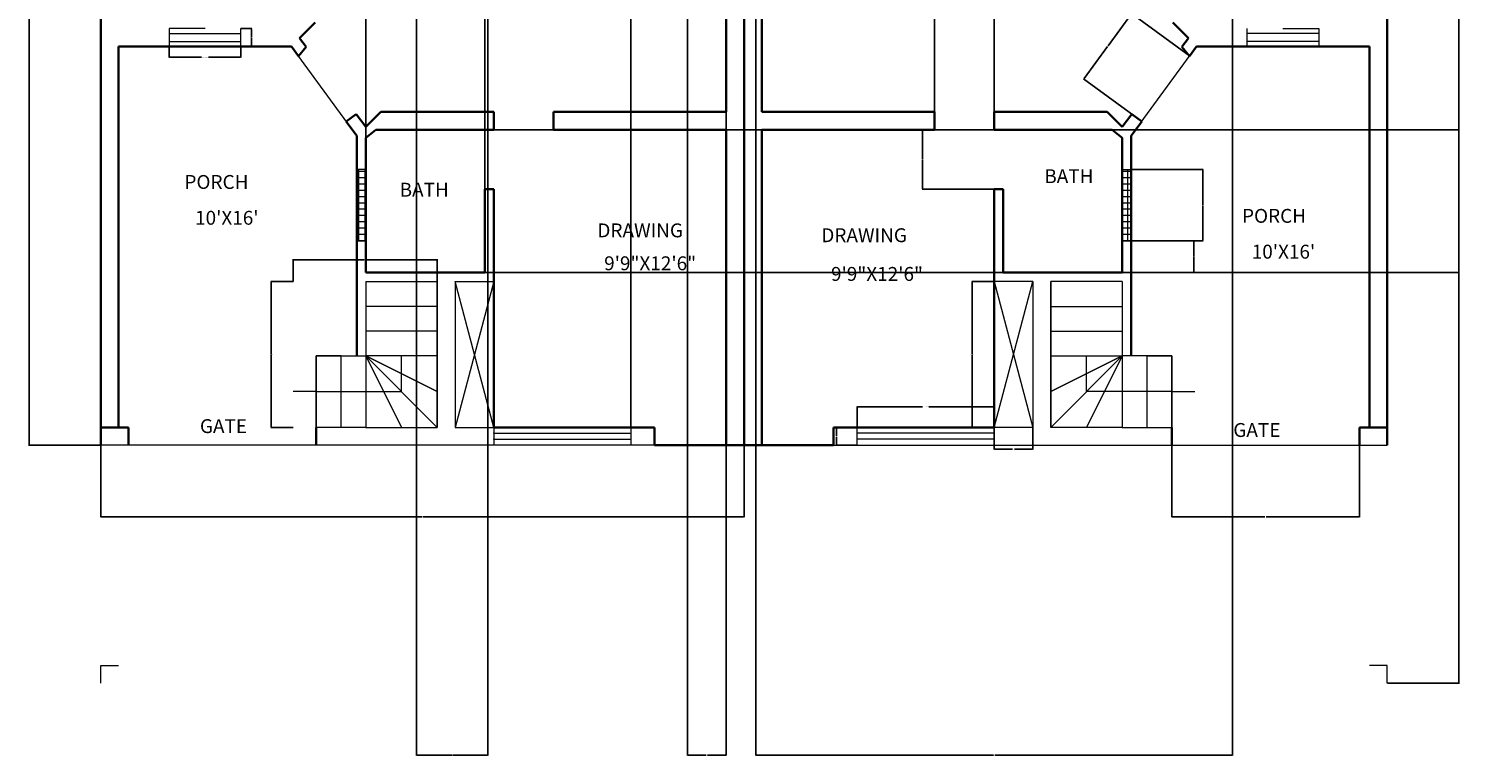
# Model space of a CAD drawing. Units: millimetres. Extents: x 2218 to 2939, y 1369 to 2162.
# Tile 1 of 2: x 2218 to 2939, y 1369 to 1736. Entities that reach past the tile are written whole.
import ezdxf

# ---------------------------------------------------------------- set-up
doc = ezdxf.new("R2010")
doc.units = ezdxf.units.MM
for name, color, linetype, lineweight in [('A-ANNO-DIMS', 2, 'Continuous', 18), ('A-ANNO-TEXT', 7, 'Continuous', 18), ('A-AREA-IDEN', 7, 'Continuous', 25), ('A-DOOR', 3, 'Continuous', 18), ('A-FLOR-CASE', 9, 'Continuous', 18), ('A-FLOR-STRS', 2, 'Continuous', 18), ('A-GLAZ', 4, 'Continuous', 18), ('A-GLAZ-PATT', 252, 'Continuous', 13), ('A-REFR-NODE', 8, 'Continuous', 13), ('A-WALL', 7, 'Continuous', 35), ('C-PROP', 8, 'Continuous', 18)]:
    doc.layers.add(name, color=color, linetype=linetype, lineweight=lineweight)
doc.styles.get("Standard").update_dxf_attribs({"font": 'arial.ttf'})
doc.dimstyles.get("Standard").update_dxf_attribs({"dimtxt": 0.18, "dimasz": 0.18, "dimexe": 0.18, "dimexo": 0.0625, "dimgap": 0.09, "dimtad": 0, "dimtih": 1, "dimtoh": 1, "dimdec": 4, "dimzin": 0, "dimdsep": 46, "dimtxsty": 'Standard', "dimcen": 0.09, "dimadec": 0, "dimazin": 0, "dimtfac": 1, "dimtdec": 4, "dimtofl": 0, "dimtmove": 0, "dimatfit": 3, "dimfxl": 1, "dimtolj": 1, "dimtzin": 0, "dimarcsym": 0})

# ---------------------------------------------------------------- blocks, each defined once
blk = doc.blocks.new('WIN-KITCHEN-PORCH')
for p, q in [((18, 9), (0, 9)), ((0, 9), (0, 0)), ((36, 0), (36, 9)), ((0, 6.5), (36, 6.5)), ((0, 2.5), (36, 2.5)), ((0, 0), (36, 0))]:
    blk.add_line(p, q)
blk = doc.blocks.new('WIN-DRAWING-FRONT')
for p, q in [((0, 9), (0, 0)), ((69, 9), (69, 0)), ((0, 6), (69, 6)), ((0, 3), (69, 3))]:
    blk.add_line(p, q)
blk = doc.blocks.new('STAIR-PORCH-WINDER')
for p, q in [((36.6, 73.5), (72.6, 73.5)), ((36.6, 73.5), (72.6, 73.5)), ((36.6, 73.5), (36.6, 0)), ((72.6, 73.5), (72.6, 0)), ((72.6, 36), (72.6, 73.5)), ((72.6, 61), (36.6, 61)), ((72.6, 48.5), (36.6, 48.5)), ((24.1, 36), (11.6, 36)), ((11.6, 36), (11.6, 0)), ((11.6, 0), (11.6, 36)), ((11.6, 36), (32.1, 36)), ((24.1, 0), (24.1, 36)), ((32.1, 36), (36.6, 36)), ((72.6, 36), (36.6, 36)), ((36.6, 36), (72.6, 18)), ((72.6, 18), (36.6, 36)), ((36.6, 36), (54.6, 0)), ((36.6, 36), (72.6, 0)), ((54.6, 18), (54.6, 36)), ((72.6, 0), (72.6, 36)), ((11.6, 18), (0, 18)), ((11.6, 18), (54.6, 18)), ((32.1, 0), (11.6, 0)), ((36.6, 0), (24.1, 0)), ((36.6, 0), (72.6, 0))]:
    blk.add_line(p, q)
blk = doc.blocks.new('CASEWORK-DRAWING')
for p, q in [((0, 73.5), (0, 0)), ((19.5, 0), (0, 73.5)), ((0, 73.5), (19.5, 73.5)), ((19.5, 73.5), (0, 0)), ((0, 73.5), (19.5, 73.5)), ((0, 0), (19.5, 0))]:
    blk.add_line(p, q)
blk = doc.blocks.new('*D15')
at = {"layer": 'A-ANNO-DIMS', "color": 0, "lineweight": -2, "transparency": 16777216}
for p, q in [((2288.88, 1726.51), (2288.88, 1721)), ((2324.88, 1726.51), (2324.88, 1721)), ((2289.06, 1721.18), (2305.18, 1721.18)), ((2324.7, 1721.18), (2308.58, 1721.18))]:
    blk.add_line(p, q, dxfattribs=at)
at = {"layer": 'A-ANNO-DIMS', "color": 0, "transparency": 16777216}
for points in [[(2289.06, 1721.21), (2289.06, 1721.15), (2288.88, 1721.18)], [(2324.7, 1721.21), (2324.7, 1721.15), (2324.88, 1721.18)]]:
    blk.add_solid(points, dxfattribs=at)
at = {"layer": 'Defpoints', "color": 0, "transparency": 16777216}
for p in [(2288.88, 1726.58), (2324.88, 1726.58), (2324.88, 1721.18)]:
    blk.add_point(p, dxfattribs=at)
at = {"layer": 'A-ANNO-DIMS', "color": 0, "transparency": 16777216, "insert": (2306.88, 1721.18), "char_height": 0.18, "attachment_point": 5}
blk.add_mtext('\\A1;KITCHEN WINDOW 36 TYP.', dxfattribs=at)
blk = doc.blocks.new('*D16')
at = {"layer": 'A-ANNO-DIMS', "color": 0, "lineweight": -2, "transparency": 16777216}
for p, q in [((2324.94, 1735.58), (2330.46, 1735.58)), ((2330.28, 1735.4), (2330.28, 1731.26)), ((2330.28, 1726.76), (2330.28, 1730.89)), ((2324.94, 1726.58), (2330.46, 1726.58))]:
    blk.add_line(p, q, dxfattribs=at)
at = {"layer": 'A-ANNO-DIMS', "color": 0, "transparency": 16777216}
for points in [[(2330.25, 1735.4), (2330.31, 1735.4), (2330.28, 1735.58)], [(2330.25, 1726.76), (2330.31, 1726.76), (2330.28, 1726.58)]]:
    blk.add_solid(points, dxfattribs=at)
at = {"layer": 'Defpoints', "color": 0, "transparency": 16777216}
for p in [(2324.88, 1735.58), (2330.28, 1735.58), (2324.88, 1726.58)]:
    blk.add_point(p, dxfattribs=at)
at = {"layer": 'A-ANNO-DIMS', "color": 0, "transparency": 16777216, "insert": (2330.28, 1731.08), "char_height": 0.18, "attachment_point": 5}
blk.add_mtext('\\A1;9 TYP.', dxfattribs=at)
blk = doc.blocks.new('*D17')
at = {"layer": 'A-ANNO-DIMS', "color": 0, "lineweight": -2, "transparency": 16777216}
for p, q in [((2635.38, 1534.64), (2635.38, 1545.11)), ((2635.56, 1544.93), (2668.3, 1544.93)), ((2704.2, 1544.93), (2671.46, 1544.93)), ((2704.38, 1534.64), (2704.38, 1545.11))]:
    blk.add_line(p, q, dxfattribs=at)
at = {"layer": 'A-ANNO-DIMS', "color": 0, "transparency": 16777216}
for points in [[(2635.56, 1544.96), (2635.56, 1544.9), (2635.38, 1544.93)], [(2704.2, 1544.96), (2704.2, 1544.9), (2704.38, 1544.93)]]:
    blk.add_solid(points, dxfattribs=at)
at = {"layer": 'Defpoints', "color": 0, "transparency": 16777216}
for p in [(2635.38, 1544.93), (2635.38, 1534.58), (2704.38, 1534.58)]:
    blk.add_point(p, dxfattribs=at)
at = {"layer": 'A-ANNO-DIMS', "color": 0, "transparency": 16777216, "insert": (2669.88, 1544.93), "char_height": 0.18, "attachment_point": 5}
blk.add_mtext('\\A1;FRONT WINDOW 69 TYP.', dxfattribs=at)
blk = doc.blocks.new('*D18')
at = {"layer": 'A-ANNO-DIMS', "color": 0, "lineweight": -2, "transparency": 16777216}
for p, q in [((2635.32, 1534.58), (2624.85, 1534.58)), ((2625.03, 1534.4), (2625.03, 1530.26)), ((2625.03, 1525.76), (2625.03, 1529.89)), ((2635.32, 1525.58), (2624.85, 1525.58))]:
    blk.add_line(p, q, dxfattribs=at)
at = {"layer": 'A-ANNO-DIMS', "color": 0, "transparency": 16777216}
for points in [[(2625, 1534.4), (2625.06, 1534.4), (2625.03, 1534.58)], [(2625, 1525.76), (2625.06, 1525.76), (2625.03, 1525.58)]]:
    blk.add_solid(points, dxfattribs=at)
at = {"layer": 'Defpoints', "color": 0, "transparency": 16777216}
for p in [(2635.38, 1534.58), (2625.03, 1525.58), (2635.38, 1525.58)]:
    blk.add_point(p, dxfattribs=at)
at = {"layer": 'A-ANNO-DIMS', "color": 0, "transparency": 16777216, "insert": (2625.03, 1530.08), "char_height": 0.18, "attachment_point": 5}
blk.add_mtext('\\A1;9 TYP.', dxfattribs=at)
blk = doc.blocks.new('*D19')
at = {"layer": 'A-ANNO-DIMS', "color": 0, "lineweight": -2, "transparency": 16777216}
for p, q in [((2351.22, 1608.08), (2340.08, 1608.08)), ((2340.26, 1607.9), (2340.26, 1571.51)), ((2340.26, 1534.76), (2340.26, 1571.14)), ((2351.22, 1534.58), (2340.08, 1534.58))]:
    blk.add_line(p, q, dxfattribs=at)
at = {"layer": 'A-ANNO-DIMS', "color": 0, "transparency": 16777216}
for points in [[(2340.23, 1607.9), (2340.29, 1607.9), (2340.26, 1608.08)], [(2340.23, 1534.76), (2340.29, 1534.76), (2340.26, 1534.58)]]:
    blk.add_solid(points, dxfattribs=at)
at = {"layer": 'Defpoints', "color": 0, "transparency": 16777216}
for p in [(2340.26, 1608.08), (2351.28, 1608.08), (2351.28, 1534.58)]:
    blk.add_point(p, dxfattribs=at)
at = {"layer": 'A-ANNO-DIMS', "color": 0, "transparency": 16777216, "insert": (2340.26, 1571.33), "char_height": 0.18, "attachment_point": 5}
blk.add_mtext('\\A1;PORCH STAIR 74 TYP.', dxfattribs=at)
blk = doc.blocks.new('*D20')
at = {"layer": 'A-ANNO-DIMS', "color": 0, "lineweight": -2, "transparency": 16777216}
for p, q in [((2351.28, 1608.14), (2351.28, 1619.28)), ((2351.46, 1619.1), (2387.05, 1619.1)), ((2423.7, 1619.1), (2388.11, 1619.1)), ((2423.88, 1608.14), (2423.88, 1619.28))]:
    blk.add_line(p, q, dxfattribs=at)
at = {"layer": 'A-ANNO-DIMS', "color": 0, "transparency": 16777216}
for points in [[(2351.46, 1619.13), (2351.46, 1619.07), (2351.28, 1619.1)], [(2423.7, 1619.13), (2423.7, 1619.07), (2423.88, 1619.1)]]:
    blk.add_solid(points, dxfattribs=at)
at = {"layer": 'Defpoints', "color": 0, "transparency": 16777216}
for p in [(2423.88, 1619.1), (2351.28, 1608.08), (2423.88, 1608.08)]:
    blk.add_point(p, dxfattribs=at)
at = {"layer": 'A-ANNO-DIMS', "color": 0, "transparency": 16777216, "insert": (2387.58, 1619.1), "char_height": 0.18, "attachment_point": 5}
blk.add_mtext('\\A1;73 TYP.', dxfattribs=at)
blk = doc.blocks.new('*D23')
at = {"layer": 'A-ANNO-DIMS', "color": 0, "lineweight": -2, "transparency": 16777216}
for p, q in [((2704.32, 1608.08), (2693.17, 1608.08)), ((2693.35, 1607.9), (2693.35, 1571.51)), ((2693.35, 1534.76), (2693.35, 1571.14)), ((2704.32, 1534.58), (2693.17, 1534.58))]:
    blk.add_line(p, q, dxfattribs=at)
at = {"layer": 'A-ANNO-DIMS', "color": 0, "transparency": 16777216}
for points in [[(2693.32, 1607.9), (2693.38, 1607.9), (2693.35, 1608.08)], [(2693.32, 1534.76), (2693.38, 1534.76), (2693.35, 1534.58)]]:
    blk.add_solid(points, dxfattribs=at)
at = {"layer": 'Defpoints', "color": 0, "transparency": 16777216}
for p in [(2693.35, 1608.08), (2704.38, 1608.08), (2704.38, 1534.58)]:
    blk.add_point(p, dxfattribs=at)
at = {"layer": 'A-ANNO-DIMS', "color": 0, "transparency": 16777216, "insert": (2693.35, 1571.33), "char_height": 0.18, "attachment_point": 5}
blk.add_mtext('\\A1;CASEWORK 74 TYP.', dxfattribs=at)
blk = doc.blocks.new('*D24')
at = {"layer": 'A-ANNO-DIMS', "color": 0, "lineweight": -2, "transparency": 16777216}
for p, q in [((2704.38, 1534.51), (2704.38, 1523.37)), ((2723.88, 1534.51), (2723.88, 1523.37)), ((2704.56, 1523.55), (2713.6, 1523.55)), ((2723.7, 1523.55), (2714.66, 1523.55))]:
    blk.add_line(p, q, dxfattribs=at)
at = {"layer": 'A-ANNO-DIMS', "color": 0, "transparency": 16777216}
for points in [[(2704.56, 1523.58), (2704.56, 1523.52), (2704.38, 1523.55)], [(2723.7, 1523.58), (2723.7, 1523.52), (2723.88, 1523.55)]]:
    blk.add_solid(points, dxfattribs=at)
at = {"layer": 'Defpoints', "color": 0, "transparency": 16777216}
for p in [(2704.38, 1534.58), (2723.88, 1534.58), (2704.38, 1523.55)]:
    blk.add_point(p, dxfattribs=at)
at = {"layer": 'A-ANNO-DIMS', "color": 0, "transparency": 16777216, "insert": (2714.13, 1523.55), "char_height": 0.18, "attachment_point": 5}
blk.add_mtext('\\A1;20 TYP.', dxfattribs=at)
blk = doc.blocks.new('*D26')
at = {"layer": 'A-ANNO-DIMS', "color": 0, "lineweight": -2, "transparency": 16777216}
for p, q in [((2254.38, 1525.51), (2254.38, 1489.25)), ((2578.38, 1525.51), (2578.38, 1489.25)), ((2254.56, 1489.43), (2416.09, 1489.43)), ((2578.2, 1489.43), (2416.67, 1489.43))]:
    blk.add_line(p, q, dxfattribs=at)
at = {"layer": 'A-ANNO-DIMS', "color": 0, "transparency": 16777216}
for points in [[(2254.56, 1489.46), (2254.56, 1489.4), (2254.38, 1489.43)], [(2578.2, 1489.46), (2578.2, 1489.4), (2578.38, 1489.43)]]:
    blk.add_solid(points, dxfattribs=at)
at = {"layer": 'Defpoints', "color": 0, "transparency": 16777216}
for p in [(2254.38, 1525.58), (2578.38, 1525.58), (2254.38, 1489.43)]:
    blk.add_point(p, dxfattribs=at)
at = {"layer": 'A-ANNO-DIMS', "color": 0, "transparency": 16777216, "insert": (2416.38, 1489.43), "char_height": 0.18, "attachment_point": 5}
blk.add_mtext('\\A1;324', dxfattribs=at)
blk = doc.blocks.new('*D27')
at = {"layer": 'A-ANNO-DIMS', "color": 0, "lineweight": -2, "transparency": 16777216}
for p, q in [((2902.44, 2125.58), (2938.71, 2125.58)), ((2938.53, 2125.4), (2938.53, 1765.76)), ((2938.53, 1405.76), (2938.53, 1765.39)), ((2902.44, 1405.58), (2938.71, 1405.58))]:
    blk.add_line(p, q, dxfattribs=at)
at = {"layer": 'A-ANNO-DIMS', "color": 0, "transparency": 16777216}
for points in [[(2938.5, 2125.4), (2938.56, 2125.4), (2938.53, 2125.58)], [(2938.5, 1405.76), (2938.56, 1405.76), (2938.53, 1405.58)]]:
    blk.add_solid(points, dxfattribs=at)
at = {"layer": 'Defpoints', "color": 0, "transparency": 16777216}
for p in [(2902.38, 2125.58), (2938.53, 2125.58), (2902.38, 1405.58)]:
    blk.add_point(p, dxfattribs=at)
at = {"layer": 'A-ANNO-DIMS', "color": 0, "transparency": 16777216, "insert": (2938.53, 1765.58), "char_height": 0.18, "attachment_point": 5}
blk.add_mtext('\\A1;720', dxfattribs=at)
blk = doc.blocks.new('*D28')
at = {"layer": 'A-ANNO-DIMS', "color": 0, "lineweight": -2, "transparency": 16777216}
for p, q in [((2254.32, 2125.58), (2218.05, 2125.58)), ((2218.23, 2125.4), (2218.23, 1825.76)), ((2218.23, 1525.76), (2218.23, 1825.39)), ((2254.32, 1525.58), (2218.05, 1525.58))]:
    blk.add_line(p, q, dxfattribs=at)
at = {"layer": 'A-ANNO-DIMS', "color": 0, "transparency": 16777216}
for points in [[(2218.2, 2125.4), (2218.26, 2125.4), (2218.23, 2125.58)], [(2218.2, 1525.76), (2218.26, 1525.76), (2218.23, 1525.58)]]:
    blk.add_solid(points, dxfattribs=at)
at = {"layer": 'Defpoints', "color": 0, "transparency": 16777216}
for p in [(2218.23, 2125.58), (2254.38, 2125.58), (2254.38, 1525.58)]:
    blk.add_point(p, dxfattribs=at)
at = {"layer": 'A-ANNO-DIMS', "color": 0, "transparency": 16777216, "insert": (2218.23, 1825.58), "char_height": 0.18, "attachment_point": 5}
blk.add_mtext('\\A1;600', dxfattribs=at)
blk = doc.blocks.new('*D29')
at = {"layer": 'A-ANNO-DIMS', "color": 0, "lineweight": -2, "transparency": 16777216}
for p, q in [((2584.38, 2119.51), (2584.38, 1369.25)), ((2824.38, 2119.51), (2824.38, 1369.25)), ((2584.56, 1369.43), (2704.09, 1369.43)), ((2824.2, 1369.43), (2704.67, 1369.43))]:
    blk.add_line(p, q, dxfattribs=at)
at = {"layer": 'A-ANNO-DIMS', "color": 0, "transparency": 16777216}
for points in [[(2584.56, 1369.46), (2584.56, 1369.4), (2584.38, 1369.43)], [(2824.2, 1369.46), (2824.2, 1369.4), (2824.38, 1369.43)]]:
    blk.add_solid(points, dxfattribs=at)
at = {"layer": 'Defpoints', "color": 0, "transparency": 16777216}
for p in [(2584.38, 2119.58), (2824.38, 2119.58), (2824.38, 1369.43)]:
    blk.add_point(p, dxfattribs=at)
at = {"layer": 'A-ANNO-DIMS', "color": 0, "transparency": 16777216, "insert": (2704.38, 1369.43), "char_height": 0.18, "attachment_point": 5}
blk.add_mtext('\\A1;240', dxfattribs=at)
blk = doc.blocks.new('*D31')
at = {"layer": 'A-ANNO-DIMS', "color": 0, "lineweight": -2, "transparency": 16777216}
for p, q in [((2387.88, 1612.64), (2387.88, 2161.91)), ((2388.06, 2161.73), (2417.66, 2161.73)), ((2447.7, 2161.73), (2418.1, 2161.73)), ((2447.88, 1612.64), (2447.88, 2161.91))]:
    blk.add_line(p, q, dxfattribs=at)
at = {"layer": 'A-ANNO-DIMS', "color": 0, "transparency": 16777216}
for points in [[(2388.06, 2161.76), (2388.06, 2161.7), (2387.88, 2161.73)], [(2447.7, 2161.76), (2447.7, 2161.7), (2447.88, 2161.73)]]:
    blk.add_solid(points, dxfattribs=at)
at = {"layer": 'Defpoints', "color": 0, "transparency": 16777216}
for p in [(2447.88, 2161.73), (2387.88, 1612.58), (2447.88, 1612.58)]:
    blk.add_point(p, dxfattribs=at)
at = {"layer": 'A-ANNO-DIMS', "color": 0, "transparency": 16777216, "insert": (2417.88, 2161.73), "char_height": 0.18, "attachment_point": 5}
blk.add_mtext('\\A1;60', dxfattribs=at)
blk = doc.blocks.new('*D32')
at = {"layer": 'A-ANNO-DIMS', "color": 0, "lineweight": -2, "transparency": 16777216}
for p, q in [((2392.94, 1684.58), (2938.71, 1684.58)), ((2938.53, 1684.4), (2938.53, 1648.76)), ((2938.53, 1612.76), (2938.53, 1648.39)), ((2387.94, 1612.58), (2938.71, 1612.58))]:
    blk.add_line(p, q, dxfattribs=at)
at = {"layer": 'A-ANNO-DIMS', "color": 0, "transparency": 16777216}
for points in [[(2938.5, 1684.4), (2938.56, 1684.4), (2938.53, 1684.58)], [(2938.5, 1612.76), (2938.56, 1612.76), (2938.53, 1612.58)]]:
    blk.add_solid(points, dxfattribs=at)
at = {"layer": 'Defpoints', "color": 0, "transparency": 16777216}
for p in [(2392.88, 1684.58), (2938.53, 1684.58), (2387.88, 1612.58)]:
    blk.add_point(p, dxfattribs=at)
at = {"layer": 'A-ANNO-DIMS', "color": 0, "transparency": 16777216, "insert": (2938.53, 1648.58), "char_height": 0.18, "attachment_point": 5}
blk.add_mtext('\\A1;72', dxfattribs=at)
blk = doc.blocks.new('*D35')
at = {"layer": 'A-ANNO-DIMS', "color": 0, "lineweight": -2, "transparency": 16777216}
for p, q in [((2549.88, 2002.51), (2549.88, 1369.25)), ((2569.38, 2002.51), (2569.38, 1369.25)), ((2550.06, 1369.43), (2559.31, 1369.43)), ((2569.2, 1369.43), (2559.95, 1369.43))]:
    blk.add_line(p, q, dxfattribs=at)
at = {"layer": 'A-ANNO-DIMS', "color": 0, "transparency": 16777216}
for points in [[(2550.06, 1369.46), (2550.06, 1369.4), (2549.88, 1369.43)], [(2569.2, 1369.46), (2569.2, 1369.4), (2569.38, 1369.43)]]:
    blk.add_solid(points, dxfattribs=at)
at = {"layer": 'Defpoints', "color": 0, "transparency": 16777216}
for p in [(2549.88, 2002.58), (2569.38, 2002.58), (2569.38, 1369.43)]:
    blk.add_point(p, dxfattribs=at)
at = {"layer": 'A-ANNO-DIMS', "color": 0, "transparency": 16777216, "insert": (2559.63, 1369.43), "char_height": 0.18, "attachment_point": 5}
blk.add_mtext('\\A1;19.5', dxfattribs=at)
blk = doc.blocks.new('*D37')
at = {"layer": 'A-ANNO-DIMS', "color": 0, "lineweight": -2, "transparency": 16777216}
for p, q in [((2521.38, 1534.64), (2521.38, 2161.91)), ((2521.56, 2161.73), (2545.16, 2161.73)), ((2569.2, 2161.73), (2545.6, 2161.73)), ((2569.38, 1525.64), (2569.38, 2161.91))]:
    blk.add_line(p, q, dxfattribs=at)
at = {"layer": 'A-ANNO-DIMS', "color": 0, "transparency": 16777216}
for points in [[(2521.56, 2161.76), (2521.56, 2161.7), (2521.38, 2161.73)], [(2569.2, 2161.76), (2569.2, 2161.7), (2569.38, 2161.73)]]:
    blk.add_solid(points, dxfattribs=at)
at = {"layer": 'Defpoints', "color": 0, "transparency": 16777216}
for p in [(2569.38, 2161.73), (2521.38, 1534.58), (2569.38, 1525.58)]:
    blk.add_point(p, dxfattribs=at)
at = {"layer": 'A-ANNO-DIMS', "color": 0, "transparency": 16777216, "insert": (2545.38, 2161.73), "char_height": 0.18, "attachment_point": 5}
blk.add_mtext('\\A1;48', dxfattribs=at)
blk = doc.blocks.new('*D38')
at = {"layer": 'A-ANNO-DIMS', "color": 0, "lineweight": -2, "transparency": 16777216}
for p, q in [((2674.38, 1693.64), (2674.38, 2161.91)), ((2674.56, 2161.73), (2689.16, 2161.73)), ((2704.2, 2161.73), (2689.6, 2161.73)), ((2704.38, 1693.64), (2704.38, 2161.91))]:
    blk.add_line(p, q, dxfattribs=at)
at = {"layer": 'A-ANNO-DIMS', "color": 0, "transparency": 16777216}
for points in [[(2674.56, 2161.76), (2674.56, 2161.7), (2674.38, 2161.73)], [(2704.2, 2161.76), (2704.2, 2161.7), (2704.38, 2161.73)]]:
    blk.add_solid(points, dxfattribs=at)
at = {"layer": 'Defpoints', "color": 0, "transparency": 16777216}
for p in [(2704.38, 2161.73), (2674.38, 1693.58), (2704.38, 1693.58)]:
    blk.add_point(p, dxfattribs=at)
at = {"layer": 'A-ANNO-DIMS', "color": 0, "transparency": 16777216, "insert": (2689.38, 2161.73), "char_height": 0.18, "attachment_point": 5}
blk.add_mtext('\\A1;30', dxfattribs=at)
blk = doc.blocks.new('*D39')
at = {"layer": 'A-ANNO-DIMS', "color": 0, "lineweight": -2, "transparency": 16777216}
for p, q in [((2413.38, 1849.51), (2413.38, 1369.25)), ((2449.38, 1849.51), (2449.38, 1369.25)), ((2413.56, 1369.43), (2431.16, 1369.43)), ((2449.2, 1369.43), (2431.6, 1369.43))]:
    blk.add_line(p, q, dxfattribs=at)
at = {"layer": 'A-ANNO-DIMS', "color": 0, "transparency": 16777216}
for points in [[(2413.56, 1369.46), (2413.56, 1369.4), (2413.38, 1369.43)], [(2449.2, 1369.46), (2449.2, 1369.4), (2449.38, 1369.43)]]:
    blk.add_solid(points, dxfattribs=at)
at = {"layer": 'Defpoints', "color": 0, "transparency": 16777216}
for p in [(2413.38, 1849.58), (2449.38, 1849.58), (2449.38, 1369.43)]:
    blk.add_point(p, dxfattribs=at)
at = {"layer": 'A-ANNO-DIMS', "color": 0, "transparency": 16777216, "insert": (2431.38, 1369.43), "char_height": 0.18, "attachment_point": 5}
blk.add_mtext('\\A1;36', dxfattribs=at)
blk = doc.blocks.new('*D40')
at = {"layer": 'A-ANNO-DIMS', "color": 0, "lineweight": -2, "transparency": 16777216}
for p, q in [((2793.88, 1525.51), (2793.88, 1489.25)), ((2888.38, 1525.51), (2888.38, 1489.25)), ((2794.06, 1489.43), (2840.8, 1489.43)), ((2888.2, 1489.43), (2841.45, 1489.43))]:
    blk.add_line(p, q, dxfattribs=at)
at = {"layer": 'A-ANNO-DIMS', "color": 0, "transparency": 16777216}
for points in [[(2794.06, 1489.46), (2794.06, 1489.4), (2793.88, 1489.43)], [(2888.2, 1489.46), (2888.2, 1489.4), (2888.38, 1489.43)]]:
    blk.add_solid(points, dxfattribs=at)
at = {"layer": 'Defpoints', "color": 0, "transparency": 16777216}
for p in [(2793.88, 1525.58), (2888.38, 1525.58), (2793.88, 1489.43)]:
    blk.add_point(p, dxfattribs=at)
at = {"layer": 'A-ANNO-DIMS', "color": 0, "transparency": 16777216, "insert": (2841.13, 1489.43), "char_height": 0.18, "attachment_point": 5}
blk.add_mtext('\\A1;94.5', dxfattribs=at)
blk = doc.blocks.new('*D44')
at = {"layer": 'A-ANNO-DIMS', "color": 0, "lineweight": -2, "transparency": 16777216}
for p, q in [((2773.57, 1742.97), (2761.75, 1726.84)), ((2802.78, 1721.77), (2773.53, 1743.22)), ((2749.66, 1710.36), (2761.48, 1726.48)), ((2778.65, 1688.87), (2749.4, 1710.32))]:
    blk.add_line(p, q, dxfattribs=at)
at = {"layer": 'A-ANNO-DIMS', "color": 0, "transparency": 16777216}
for points in [[(2773.55, 1742.99), (2773.6, 1742.95), (2773.68, 1743.11)], [(2749.63, 1710.37), (2749.68, 1710.34), (2749.55, 1710.21)]]:
    blk.add_solid(points, dxfattribs=at)
at = {"layer": 'Defpoints', "color": 0, "transparency": 16777216}
for p in [(2773.68, 1743.11), (2802.83, 1721.74), (2778.7, 1688.83)]:
    blk.add_point(p, dxfattribs=at)
at = {"layer": 'A-ANNO-DIMS', "color": 0, "transparency": 16777216, "insert": (2761.61, 1726.66), "char_height": 0.18, "attachment_point": 5}
blk.add_mtext('\\A1;40.8', dxfattribs=at)
blk = doc.blocks.new('*D45')
at = {"layer": 'A-ANNO-DIMS', "color": 0, "lineweight": -2, "transparency": 16777216}
for p, q in [((2773.44, 1664.58), (2809.71, 1664.58)), ((2809.53, 1664.4), (2809.53, 1646.76)), ((2809.53, 1628.76), (2809.53, 1646.39)), ((2773.44, 1628.58), (2809.71, 1628.58))]:
    blk.add_line(p, q, dxfattribs=at)
at = {"layer": 'A-ANNO-DIMS', "color": 0, "transparency": 16777216}
for points in [[(2809.5, 1664.4), (2809.56, 1664.4), (2809.53, 1664.58)], [(2809.5, 1628.76), (2809.56, 1628.76), (2809.53, 1628.58)]]:
    blk.add_solid(points, dxfattribs=at)
at = {"layer": 'Defpoints', "color": 0, "transparency": 16777216}
for p in [(2773.38, 1664.58), (2773.38, 1628.58), (2809.53, 1628.58)]:
    blk.add_point(p, dxfattribs=at)
at = {"layer": 'A-ANNO-DIMS', "color": 0, "transparency": 16777216, "insert": (2809.53, 1646.58), "char_height": 0.18, "attachment_point": 5}
blk.add_mtext('\\A1;36', dxfattribs=at)
blk = doc.blocks.new('*D46')
at = {"layer": 'A-ANNO-DIMS', "color": 0, "lineweight": -2, "transparency": 16777216}
for p, q in [((2768.94, 1628.58), (2805.21, 1628.58)), ((2805.03, 1628.4), (2805.03, 1620.76)), ((2805.03, 1612.76), (2805.03, 1620.39)), ((2768.94, 1612.58), (2805.21, 1612.58))]:
    blk.add_line(p, q, dxfattribs=at)
at = {"layer": 'A-ANNO-DIMS', "color": 0, "transparency": 16777216}
for points in [[(2805, 1628.4), (2805.06, 1628.4), (2805.03, 1628.58)], [(2805, 1612.76), (2805.06, 1612.76), (2805.03, 1612.58)]]:
    blk.add_solid(points, dxfattribs=at)
at = {"layer": 'Defpoints', "color": 0, "transparency": 16777216}
for p in [(2768.88, 1628.58), (2768.88, 1612.58), (2805.03, 1612.58)]:
    blk.add_point(p, dxfattribs=at)
at = {"layer": 'A-ANNO-DIMS', "color": 0, "transparency": 16777216, "insert": (2805.03, 1620.58), "char_height": 0.18, "attachment_point": 5}
blk.add_mtext('\\A1;16', dxfattribs=at)
blk = doc.blocks.new('*D47')
at = {"layer": 'A-ANNO-DIMS', "color": 0, "lineweight": -2, "transparency": 16777216}
for p, q in [((2704.32, 1684.58), (2668.05, 1684.58)), ((2668.23, 1684.4), (2668.23, 1669.76)), ((2668.23, 1654.76), (2668.23, 1669.39)), ((2704.32, 1654.58), (2668.05, 1654.58))]:
    blk.add_line(p, q, dxfattribs=at)
at = {"layer": 'A-ANNO-DIMS', "color": 0, "transparency": 16777216}
for points in [[(2668.2, 1684.4), (2668.26, 1684.4), (2668.23, 1684.58)], [(2668.2, 1654.76), (2668.26, 1654.76), (2668.23, 1654.58)]]:
    blk.add_solid(points, dxfattribs=at)
at = {"layer": 'Defpoints', "color": 0, "transparency": 16777216}
for p in [(2668.23, 1684.58), (2704.38, 1684.58), (2704.38, 1654.58)]:
    blk.add_point(p, dxfattribs=at)
at = {"layer": 'A-ANNO-DIMS', "color": 0, "transparency": 16777216, "insert": (2668.23, 1669.58), "char_height": 0.18, "attachment_point": 5}
blk.add_mtext('\\A1;30', dxfattribs=at)

msp = doc.modelspace()

# ---------------------------------------------------------------- hatches: boundary and pattern name
at = {"layer": 'A-GLAZ-PATT'}
h = msp.add_hatch(dxfattribs=at)
h.set_pattern_fill('NET', color=256)
h.paths.add_polyline_path([(2387.88, 1646.58), (2387.88, 1664.58), (2383.38, 1664.58), (2383.38, 1628.58), (2387.88, 1628.58)])
h = msp.add_hatch(dxfattribs=at)
h.set_pattern_fill('NET', color=256)
h.paths.add_polyline_path([(2768.88, 1646.58), (2768.88, 1664.58), (2773.38, 1664.58), (2773.38, 1628.58), (2768.88, 1628.58)])

# ---------------------------------------------------------------- linework, layer by layer
at = {"layer": 'A-DOOR'}
for p, q in [((2383.38, 1681.58), (2350.38, 1726.58)), ((2773.38, 1681.58), (2806.38, 1726.58))]:
    msp.add_line(p, q, dxfattribs=at)
at = {"layer": 'A-GLAZ'}
for p, q in [((2387.88, 1664.58), (2383.38, 1664.58)), ((2383.38, 1664.58), (2383.38, 1628.58)), ((2387.88, 1646.58), (2387.88, 1664.58)), ((2768.88, 1646.58), (2768.88, 1664.58)), ((2768.88, 1664.58), (2773.38, 1664.58)), ((2773.38, 1664.58), (2773.38, 1628.58)), ((2383.38, 1628.58), (2387.88, 1628.58)), ((2773.38, 1628.58), (2768.88, 1628.58))]:
    msp.add_line(p, q, dxfattribs=at)
at = {"layer": 'A-REFR-NODE'}
for p in [(2423.88, 1595.58), (2732.88, 1595.58), (2423.88, 1583.08), (2732.88, 1583.08), (2452.38, 1531.58), (2452.38, 1528.58), (2704.38, 1531.58), (2704.38, 1528.58)]:
    msp.add_point(p, dxfattribs=at)
at = {"layer": 'A-WALL'}
for p, q in [((2254.38, 2125.58), (2254.38, 1525.58)), ((2578.38, 2125.58), (2578.38, 1525.58)), ((2578.38, 2125.58), (2578.38, 1525.58)), ((2902.38, 2125.58), (2902.38, 1525.58)), ((2569.38, 1695.08), (2569.38, 1851.08)), ((2587.38, 1695.08), (2587.38, 1851.08)), ((2354.53, 1730.72), (2362.38, 1738.58)), ((2802.23, 1730.72), (2794.38, 1738.58)), ((2357.8, 1726.33), (2354.53, 1730.72)), ((2798.96, 1726.33), (2802.23, 1730.72)), ((2263.38, 1534.58), (2263.38, 1726.58)), ((2263.38, 1726.58), (2350.38, 1726.58)), ((2263.38, 1534.58), (2263.38, 1726.58)), ((2350.38, 1726.58), (2353.93, 1721.74)), ((2353.93, 1721.74), (2350.38, 1726.58)), ((2353.93, 1721.74), (2357.8, 1726.33)), ((2802.83, 1721.74), (2798.96, 1726.33)), ((2802.83, 1721.74), (2806.38, 1726.58)), ((2806.38, 1726.58), (2802.83, 1721.74)), ((2893.38, 1726.58), (2806.38, 1726.58)), ((2893.38, 1534.58), (2893.38, 1726.58)), ((2893.38, 1534.58), (2893.38, 1726.58)), ((2569.38, 1695.08), (2569.38, 1693.58)), ((2587.38, 1695.08), (2587.38, 1693.58)), ((2378.06, 1688.83), (2382.99, 1692.5)), ((2383.38, 1681.58), (2378.06, 1688.83)), ((2383.38, 1681.58), (2378.06, 1688.83)), ((2387.82, 1686.01), (2382.99, 1692.5)), ((2387.82, 1686.01), (2395.38, 1693.58)), ((2395.38, 1693.58), (2452.38, 1693.58)), ((2452.38, 1684.58), (2452.38, 1693.58)), ((2482.38, 1693.58), (2482.38, 1684.58)), ((2482.38, 1693.58), (2569.38, 1693.58)), ((2674.38, 1693.58), (2587.38, 1693.58)), ((2674.38, 1693.58), (2674.38, 1684.58)), ((2761.38, 1693.58), (2704.38, 1693.58)), ((2704.38, 1684.58), (2704.38, 1693.58)), ((2768.94, 1686.01), (2761.38, 1693.58)), ((2768.94, 1686.01), (2773.77, 1692.5)), ((2773.38, 1681.58), (2778.7, 1688.83)), ((2773.38, 1681.58), (2778.7, 1688.83)), ((2778.7, 1688.83), (2773.77, 1692.5)), ((2383.38, 1681.58), (2383.38, 1570.58)), ((2387.88, 1680.58), (2392.88, 1684.58)), ((2387.88, 1612.58), (2387.88, 1680.58)), ((2387.88, 1680.58), (2387.88, 1612.58)), ((2392.88, 1684.58), (2447.88, 1684.58)), ((2452.38, 1684.58), (2447.88, 1684.58)), ((2569.38, 1684.58), (2482.38, 1684.58)), ((2569.38, 1534.58), (2569.38, 1684.58)), ((2587.38, 1684.58), (2674.38, 1684.58)), ((2587.38, 1534.58), (2587.38, 1684.58)), ((2704.38, 1684.58), (2708.88, 1684.58)), ((2763.88, 1684.58), (2708.88, 1684.58)), ((2768.88, 1680.58), (2763.88, 1684.58)), ((2768.88, 1612.58), (2768.88, 1680.58)), ((2768.88, 1680.58), (2768.88, 1612.58)), ((2773.38, 1681.58), (2773.38, 1570.58)), ((2447.88, 1654.58), (2447.88, 1612.58)), ((2452.38, 1654.58), (2447.88, 1654.58)), ((2452.38, 1654.58), (2452.38, 1536.08)), ((2452.38, 1654.58), (2452.38, 1534.58)), ((2704.38, 1654.58), (2704.38, 1536.08)), ((2704.38, 1654.58), (2704.38, 1534.58)), ((2704.38, 1654.58), (2708.88, 1654.58)), ((2708.88, 1654.58), (2708.88, 1612.58)), ((2387.88, 1612.58), (2387.88, 1646.58)), ((2768.88, 1612.58), (2768.88, 1646.58)), ((2447.88, 1612.58), (2387.88, 1612.58)), ((2452.38, 1612.58), (2452.38, 1608.08)), ((2704.38, 1612.58), (2704.38, 1608.08)), ((2708.88, 1612.58), (2768.88, 1612.58)), ((2254.38, 1525.58), (2254.38, 1534.58)), ((2254.38, 1534.58), (2263.38, 1534.58)), ((2254.38, 1534.58), (2263.38, 1534.58)), ((2263.38, 1534.58), (2266.38, 1534.58)), ((2268.38, 1534.58), (2263.38, 1534.58)), ((2266.38, 1534.58), (2268.38, 1534.58)), ((2268.38, 1534.58), (2268.38, 1525.58)), ((2362.88, 1534.58), (2362.88, 1525.58)), ((2452.38, 1534.58), (2533.38, 1534.58)), ((2533.38, 1534.58), (2521.38, 1534.58)), ((2533.38, 1534.58), (2533.38, 1525.58)), ((2569.38, 1525.58), (2569.38, 1534.58)), ((2587.38, 1525.58), (2587.38, 1534.58)), ((2704.38, 1534.58), (2623.38, 1534.58)), ((2623.38, 1534.58), (2623.38, 1525.58)), ((2623.38, 1534.58), (2635.38, 1534.58)), ((2793.88, 1534.58), (2793.88, 1525.58)), ((2888.38, 1534.58), (2893.38, 1534.58)), ((2890.38, 1534.58), (2888.38, 1534.58)), ((2888.38, 1534.58), (2888.38, 1525.58)), ((2893.38, 1534.58), (2890.38, 1534.58)), ((2902.38, 1534.58), (2893.38, 1534.58)), ((2902.38, 1534.58), (2893.38, 1534.58)), ((2902.38, 1525.58), (2902.38, 1534.58)), ((2533.38, 1525.58), (2578.38, 1525.58)), ((2578.38, 1525.58), (2569.38, 1525.58)), ((2623.38, 1525.58), (2578.38, 1525.58)), ((2578.38, 1525.58), (2587.38, 1525.58))]:
    msp.add_line(p, q, dxfattribs=at)
at = {"layer": 'C-PROP'}
for p, q in [((2578.38, 1525.58), (2254.38, 1525.58)), ((2578.38, 1525.58), (2902.38, 1525.58)), ((2254.38, 1405.58), (2254.38, 1414.58)), ((2254.38, 1414.58), (2263.38, 1414.58)), ((2902.38, 1414.58), (2893.38, 1414.58)), ((2902.38, 1405.58), (2902.38, 1414.58))]:
    msp.add_line(p, q, dxfattribs=at)

# ---------------------------------------------------------------- block references
at = {"layer": 'A-FLOR-CASE'}
msp.add_blockref('CASEWORK-DRAWING', (2432.88, 1534.58), dxfattribs=at)
at = {"layer": 'A-FLOR-CASE', "extrusion": (0, 0, -1), "zscale": -1}
msp.add_blockref('CASEWORK-DRAWING', (-2723.88, 1534.58), dxfattribs=at)
at = {"layer": 'A-FLOR-STRS'}
msp.add_blockref('STAIR-PORCH-WINDER', (2351.28, 1534.58), dxfattribs=at)
at = {"layer": 'A-FLOR-STRS', "extrusion": (0, 0, -1), "zscale": -1}
msp.add_blockref('STAIR-PORCH-WINDER', (-2805.48, 1534.58), dxfattribs=at)
at = {"layer": 'A-GLAZ'}
for name, p in [('WIN-KITCHEN-PORCH', (2288.88, 1726.58)), ('WIN-DRAWING-FRONT', (2452.38, 1525.58))]:
    msp.add_blockref(name, p, dxfattribs=at)
at = {"layer": 'A-GLAZ', "extrusion": (0, 0, -1), "zscale": -1}
msp.add_blockref('WIN-KITCHEN-PORCH', (-2867.88, 1726.58), dxfattribs=at)
at = {"layer": 'A-GLAZ', "rotation": 180}
msp.add_blockref('WIN-DRAWING-FRONT', (2704.38, 1534.58), dxfattribs=at)

# ---------------------------------------------------------------- texts
at = {"layer": 'A-ANNO-DIMS'}
for s, p in [("10'X16'", (2301.88, 1636.72)), ("10'X16'", (2834.14, 1619.64)), ('9\'9"X12\'6"', (2507.94, 1613.78)), ('9\'9"X12\'6"', (2622.21, 1608.42))]:
    msp.add_text(s, height=7, dxfattribs=at).set_placement(p)
at = {"layer": 'A-ANNO-TEXT'}
for p in [(2304.32, 1531.71), (2824.86, 1529.76)]:
    msp.add_text('GATE', height=7, dxfattribs=at).set_placement(p)
at = {"layer": 'A-AREA-IDEN'}
for s, p in [('PORCH', (2296.51, 1654.77)), ('BATH', (2404.91, 1650.87)), ('BATH', (2729.64, 1657.7)), ('PORCH', (2829.25, 1637.69)), ('DRAWING', (2504.53, 1630.37)), ('DRAWING', (2617.33, 1627.93))]:
    msp.add_text(s, height=7, dxfattribs=at).set_placement(p)

# ---------------------------------------------------------------- dimensions: what is measured, and where the dimension line sits
at = {"layer": 'A-ANNO-DIMS'}
for base, p1, p2, override, picture, middle in [((2447.88, 2161.73), (2387.88, 1612.58), (2447.88, 1612.58), {"dimdec": 0, "dimlfac": 1, "dimrnd": 0, "dimzin": 0, "dimdsep": 46, "dimlunit": 2}, '*D31', (2417.88, 2161.73)), ((2569.38, 2161.73), (2521.38, 1534.58), (2569.38, 1525.58), {"dimdec": 0, "dimlfac": 1, "dimrnd": 0, "dimzin": 0, "dimdsep": 46, "dimlunit": 2}, '*D37', (2545.38, 2161.73)), ((2704.38, 2161.73), (2674.38, 1693.58), (2704.38, 1693.58), {"dimdec": 0, "dimlfac": 1, "dimrnd": 0, "dimzin": 0, "dimdsep": 46, "dimlunit": 2}, '*D38', (2689.38, 2161.73)), ((2824.38, 1369.43), (2584.38, 2119.58), (2824.38, 2119.58), {"dimdec": 0, "dimlfac": 1, "dimrnd": 0, "dimzin": 0, "dimdsep": 46, "dimlunit": 2}, '*D29', (2704.38, 1369.43)), ((2569.38, 1369.43), (2549.88, 2002.58), (2569.38, 2002.58), {"dimdec": 1, "dimlfac": 1, "dimrnd": 0, "dimzin": 0, "dimdsep": 46, "dimlunit": 2}, '*D35', (2559.63, 1369.43)), ((2449.38, 1369.43), (2413.38, 1849.58), (2449.38, 1849.58), {"dimdec": 0, "dimlfac": 1, "dimrnd": 0, "dimzin": 0, "dimdsep": 46, "dimlunit": 2}, '*D39', (2431.38, 1369.43))]:
    dim = msp.add_linear_dim(base=base, p1=p1, p2=p2, dimstyle='Standard', override=override, dxfattribs=at)
    dim.commit()
    dim.dimension.update_dxf_attribs({"geometry": picture, "text_midpoint": middle})
for base, p1, p2, angle, override, picture, middle in [((2218.23, 2125.58), (2254.38, 1525.58), (2254.38, 2125.58), 90, {"dimdec": 0, "dimlfac": 1, "dimrnd": 0, "dimzin": 0, "dimdsep": 46, "dimlunit": 2}, '*D28', (2218.23, 1825.58)), ((2938.53, 2125.58), (2902.38, 1405.58), (2902.38, 2125.58), 90, {"dimdec": 0, "dimlfac": 1, "dimrnd": 0, "dimzin": 0, "dimdsep": 46, "dimlunit": 2}, '*D27', (2938.53, 1765.58)), ((2773.68, 1743.11), (2778.7, 1688.83), (2802.83, 1721.74), 53.74616, {"dimdec": 1, "dimlfac": 1, "dimrnd": 0, "dimzin": 0, "dimdsep": 46, "dimlunit": 2}, '*D44', (2761.61, 1726.66)), ((2938.53, 1684.58), (2387.88, 1612.58), (2392.88, 1684.58), 90, {"dimdec": 0, "dimlfac": 1, "dimrnd": 0, "dimzin": 0, "dimdsep": 46, "dimlunit": 2}, '*D32', (2938.53, 1648.58)), ((2668.23, 1684.58), (2704.38, 1654.58), (2704.38, 1684.58), 90, {"dimdec": 0, "dimlfac": 1, "dimrnd": 0, "dimzin": 0, "dimdsep": 46, "dimlunit": 2}, '*D47', (2668.23, 1669.58)), ((2809.53, 1628.58), (2773.38, 1664.58), (2773.38, 1628.58), 270, {"dimdec": 0, "dimlfac": 1, "dimrnd": 0, "dimzin": 0, "dimdsep": 46, "dimlunit": 2}, '*D45', (2809.53, 1646.58)), ((2805.03, 1612.58), (2768.88, 1628.58), (2768.88, 1612.58), 270, {"dimdec": 0, "dimlfac": 1, "dimrnd": 0, "dimzin": 0, "dimdsep": 46, "dimlunit": 2}, '*D46', (2805.03, 1620.58)), ((2254.38, 1489.43), (2578.38, 1525.58), (2254.38, 1525.58), 180, {"dimdec": 0, "dimlfac": 1, "dimrnd": 0, "dimzin": 0, "dimdsep": 46, "dimlunit": 2}, '*D26', (2416.38, 1489.43)), ((2793.88, 1489.43), (2888.38, 1525.58), (2793.88, 1525.58), 180, {"dimdec": 1, "dimlfac": 1, "dimrnd": 0, "dimzin": 0, "dimdsep": 46, "dimlunit": 2}, '*D40', (2841.13, 1489.43))]:
    dim = msp.add_linear_dim(base=base, p1=p1, p2=p2, angle=angle, dimstyle='Standard', override=override, dxfattribs=at)
    dim.commit()
    dim.dimension.update_dxf_attribs({"geometry": picture, "text_midpoint": middle})
for base, p1, p2, angle, text, picture, middle in [((2330.28, 1735.58), (2324.88, 1726.58), (2324.88, 1735.58), 90, '<> TYP.', '*D16', (2330.28, 1731.08)), ((2340.25722155, 1608.07532199), (2351.28222155, 1534.57532199), (2351.28222155, 1608.07532199), 90, 'PORCH STAIR <> TYP.', '*D19', (2340.25722155, 1571.32532199)), ((2693.35423682, 1608.07532199), (2704.37923682, 1534.57532199), (2704.37923682, 1608.07532199), 90, 'CASEWORK <> TYP.', '*D23', (2693.35423682, 1571.32532199)), ((2635.38, 1544.93), (2704.38, 1534.58), (2635.38, 1534.58), 180, 'FRONT WINDOW <> TYP.', '*D17', (2669.88, 1544.93)), ((2625.03, 1525.58), (2635.38, 1534.58), (2635.38, 1525.58), 270, '<> TYP.', '*D18', (2625.03, 1530.08)), ((2704.37923682, 1523.55032199), (2723.87923682, 1534.57532199), (2704.37923682, 1534.57532199), 180, '<> TYP.', '*D24', (2714.12923682, 1523.55032199))]:
    dim = msp.add_linear_dim(base=base, p1=p1, p2=p2, angle=angle, text=text, dimstyle='Standard', override={"dimdec": 0, "dimlfac": 1, "dimrnd": 0, "dimzin": 0, "dimdsep": 46, "dimlunit": 2}, dxfattribs=at)
    dim.commit()
    dim.dimension.update_dxf_attribs({"geometry": picture, "text_midpoint": middle})
for base, p1, p2, text, picture, middle in [((2324.88, 1721.18), (2288.88, 1726.58), (2324.88, 1726.58), 'KITCHEN WINDOW <> TYP.', '*D15', (2306.88, 1721.18)), ((2423.88, 1619.1), (2351.28, 1608.08), (2423.88, 1608.08), '<> TYP.', '*D20', (2387.58, 1619.1))]:
    dim = msp.add_linear_dim(base=base, p1=p1, p2=p2, text=text, dimstyle='Standard', override={"dimdec": 0, "dimlfac": 1, "dimrnd": 0, "dimzin": 0, "dimdsep": 46, "dimlunit": 2}, dxfattribs=at)
    dim.commit()
    dim.dimension.update_dxf_attribs({"geometry": picture, "text_midpoint": middle})

doc.saveas('drawing.dxf')
